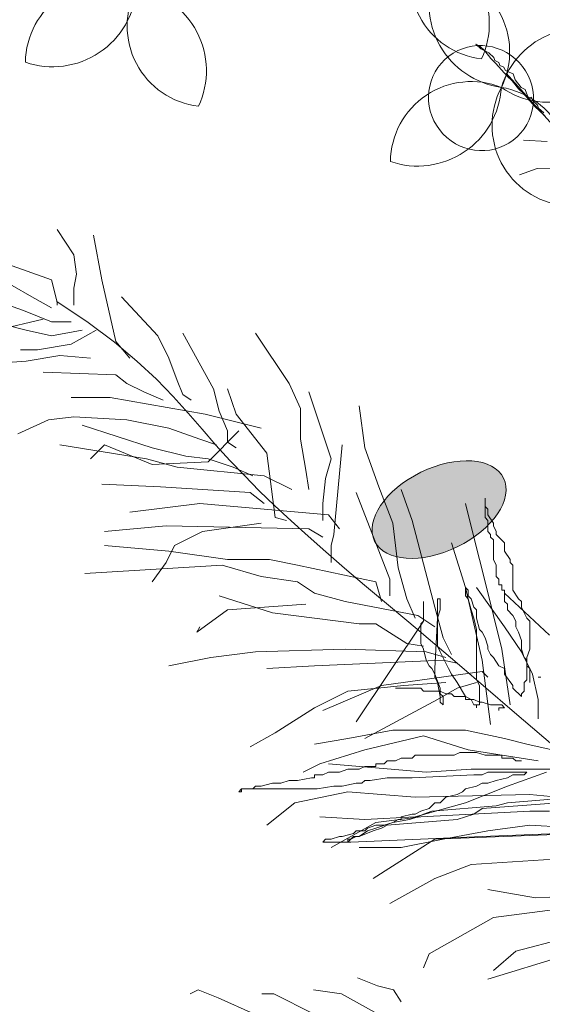
# Model space of a CAD drawing. Units: millimetres. Extents: x 595116 to 630915, y 909473 to 920225.
# Tile 100 of 134: x 629798.317 to 629803.095, y 919172.019 to 919181.018. Entities that reach past the tile are written whole.
import ezdxf

# ---------------------------------------------------------------- set-up
doc = ezdxf.new("R2010")
doc.units = ezdxf.units.MM
doc.layers.add('L-PLNT', color=85, linetype='Continuous', lineweight=13)

# ---------------------------------------------------------------- blocks, each defined once
blk = doc.blocks.new('A$C4FB75ABC')
for p, q in [((1.9382, 4.6431), (1.9285, 4.6477)), ((1.9285, 4.6477), (1.9408, 4.6359)), ((1.9506, 4.6313), (1.9382, 4.6431)), ((1.9408, 4.6359), (1.9506, 4.6313)), ((1.9603, 4.6267), (1.9506, 4.6313)), ((1.9506, 4.6313), (1.9655, 4.6124)), ((1.9726, 4.6149), (1.9603, 4.6267)), ((1.9655, 4.6124), (1.9778, 4.6006)), ((1.9752, 4.6078), (1.9726, 4.6149)), ((1.985, 4.6032), (1.9752, 4.6078)), ((1.9876, 4.596), (1.985, 4.6032)), ((1.9778, 4.6006), (2.0051, 4.5699)), ((1.9973, 4.5914), (1.9876, 4.596)), ((1.9999, 4.5842), (1.9973, 4.5914)), ((2.0097, 4.5796), (1.9999, 4.5842)), ((2.0194, 4.575), (2.0097, 4.5796)), ((2.1238, 4.4424), (2.0025, 4.577)), ((2.0051, 4.5699), (2.0174, 4.5581)), ((2.0174, 4.5581), (2.0323, 4.5391)), ((2.0246, 4.5607), (2.0194, 4.575)), ((2.0395, 4.5417), (2.0246, 4.5607)), ((2.0323, 4.5391), (2.0447, 4.5274)), ((2.0493, 4.5371), (2.0395, 4.5417)), ((2.057, 4.5156), (2.0493, 4.5371)), ((2.0447, 4.5274), (2.0719, 4.4967)), ((2.0642, 4.5182), (2.057, 4.5156)), ((2.0668, 4.511), (2.0642, 4.5182)), ((2.0791, 4.4992), (2.0668, 4.511)), ((2.0719, 4.4967), (2.0966, 4.4731)), ((2.0817, 4.4921), (2.0791, 4.4992)), ((2.094, 4.4803), (2.0817, 4.4921)), ((2.1029, 4.4105), (2.0449, 4.414)), ((2.0779, 4.3448), (2.0349, 4.3293)), ((2.1261, 4.346), (2.0779, 4.3448)), ((0.9087, 4.1962), (0.9496, 4.1349)), ((0.9973, 4.1826), (1.0177, 4.0736)), ((0.9496, 4.1349), (0.9564, 4.0872)), ((0.7997, 4.1076), (0.8951, 4.0736)), ((0.9564, 4.0872), (0.9496, 4.0532)), ((0.8474, 4.0327), (0.7997, 4.06)), ((0.8951, 4.0736), (0.9087, 4.0191)), ((0.9496, 4.0532), (0.9496, 4.0123)), ((1.0177, 4.0736), (1.0518, 3.9238)), ((0.8951, 4.0055), (0.8474, 4.0327)), ((1.0654, 4.0327), (1.154, 3.9374)), ((0.752, 4.0259), (0.827, 3.9987)), ((0.9842, 3.9699), (0.9085, 4.0207)), ((0.9087, 4.0191), (0.9087, 4.0123)), ((0.827, 3.9987), (0.8951, 3.9715)), ((0.8746, 3.9783), (0.7316, 3.9442)), ((0.8338, 3.951), (0.7793, 3.9647)), ((0.8951, 3.9715), (0.9428, 3.9715)), ((1.0487, 3.9217), (0.9842, 3.9699)), ((0.8951, 3.9374), (0.8338, 3.951)), ((0.97, 3.951), (0.8951, 3.9374)), ((1.0041, 3.951), (0.9428, 3.917)), ((1.154, 3.9374), (1.1812, 3.8829)), ((1.2153, 3.9442), (1.2902, 3.808)), ((1.3924, 3.9442), (1.4742, 3.8217)), ((0.9428, 3.917), (0.861, 3.9034)), ((1.1035, 3.8758), (1.0487, 3.9217)), ((1.0518, 3.9238), (1.0858, 3.8829)), ((0.861, 3.9034), (0.8201, 3.9034)), ((0.9155, 3.8897), (0.8338, 3.8761)), ((0.9905, 3.8829), (0.9155, 3.8897)), ((0.8338, 3.8761), (0.7452, 3.8693)), ((1.1506, 3.8319), (1.1035, 3.8758)), ((1.1812, 3.8829), (1.2017, 3.8285)), ((0.8746, 3.8489), (1.0518, 3.8421)), ((1.0518, 3.8421), (1.079, 3.8217)), ((1.079, 3.8217), (1.1199, 3.8012)), ((1.1917, 3.7897), (1.1506, 3.8319)), ((1.2017, 3.8285), (1.2153, 3.7944)), ((1.4742, 3.8217), (1.5014, 3.7604)), ((1.1199, 3.8012), (1.1676, 3.7808)), ((1.2284, 3.7492), (1.1917, 3.7897)), ((1.2153, 3.7944), (1.2357, 3.7808)), ((1.2902, 3.808), (1.3039, 3.7536)), ((1.3243, 3.808), (1.3447, 3.7467)), ((1.5219, 3.8012), (1.5764, 3.6378)), ((0.9428, 3.7876), (1.0382, 3.7876)), ((1.0382, 3.7876), (1.2698, 3.7467)), ((1.6445, 3.7672), (1.6581, 3.665)), ((1.2625, 3.7099), (1.2284, 3.7492)), ((1.2698, 3.7467), (1.4061, 3.7127)), ((1.3039, 3.7536), (1.3243, 3.7059)), ((1.3447, 3.7467), (1.4197, 3.6514)), ((1.5014, 3.7604), (1.5014, 3.6855)), ((0.8133, 3.6991), (0.8883, 3.7331)), ((0.8883, 3.7331), (0.9496, 3.7399)), ((0.9496, 3.7399), (1.079, 3.7331)), ((0.97, 3.7195), (1.1403, 3.665)), ((1.079, 3.7331), (1.1812, 3.7127)), ((1.1812, 3.7127), (1.2562, 3.6855)), ((1.2959, 3.6716), (1.2625, 3.7099)), ((1.3515, 3.7059), (1.2766, 3.631)), ((1.3243, 3.7059), (1.3243, 3.6787)), ((0.9155, 3.6718), (1.1267, 3.6378)), ((1.0245, 3.6718), (0.9905, 3.6378)), ((1.1403, 3.6242), (1.0245, 3.6718)), ((1.2562, 3.6855), (1.297, 3.6718)), ((1.3299, 3.6341), (1.2959, 3.6716)), ((1.3243, 3.6787), (1.3447, 3.665)), ((1.5014, 3.6855), (1.5151, 3.6106)), ((1.6036, 3.6718), (1.5832, 3.4539)), ((1.1403, 3.665), (1.2221, 3.6446)), ((1.2221, 3.6446), (1.2766, 3.6378)), ((1.4197, 3.6514), (1.4401, 3.4948)), ((1.6581, 3.665), (1.6922, 3.5697)), ((1.1267, 3.6378), (1.2017, 3.6174)), ((1.2766, 3.631), (1.1403, 3.6242)), ((1.2766, 3.6378), (1.3379, 3.6174)), ((1.365, 3.5971), (1.3299, 3.6341)), ((1.5764, 3.6378), (1.5627, 3.5901)), ((1.2017, 3.6174), (1.4129, 3.5969)), ((1.3379, 3.6174), (1.3856, 3.5969)), ((1.4014, 3.5604), (1.365, 3.5971)), ((1.4129, 3.5969), (1.481, 3.5629)), ((1.5151, 3.6106), (1.5219, 3.5629)), ((1.0177, 3.5765), (1.1608, 3.5697)), ((1.5627, 3.5901), (1.5559, 3.5288)), ((1.1608, 3.5697), (1.3788, 3.5561)), ((1.3788, 3.5561), (1.4129, 3.5288)), ((1.4393, 3.5237), (1.4014, 3.5604)), ((1.6377, 3.5561), (1.7194, 3.345)), ((1.6922, 3.5697), (1.7263, 3.4812)), ((1.7467, 3.5629), (1.7739, 3.488)), ((1.0858, 3.5084), (1.2562, 3.5288)), ((1.2562, 3.5288), (1.5696, 3.5016)), ((1.5559, 3.5288), (1.5559, 3.488)), ((1.9034, 3.5288), (1.9238, 3.4471)), ((1.9511, 3.4948), (1.9511, 3.5425)), ((1.9511, 3.5425), (1.9511, 3.522)), ((1.4788, 3.4868), (1.4393, 3.5237)), ((1.5696, 3.5016), (1.5968, 3.4676)), ((1.9511, 3.522), (1.9579, 3.5152)), ((1.9579, 3.5152), (1.9579, 3.5016)), ((1.9579, 3.5016), (1.9715, 3.4812)), ((1.4061, 3.4812), (1.263, 3.4608)), ((1.4401, 3.4948), (1.4674, 3.488)), ((1.5201, 3.4494), (1.4788, 3.4868)), ((1.7263, 3.4812), (1.7399, 3.3722)), ((1.7739, 3.488), (1.8285, 3.2769)), ((1.9579, 3.488), (1.9511, 3.4948)), ((1.9579, 3.4608), (1.9579, 3.488)), ((1.9715, 3.4812), (1.9715, 3.4744)), ((1.0245, 3.4608), (1.1744, 3.4744)), ((1.1744, 3.4744), (1.5219, 3.4676)), ((1.263, 3.4608), (1.1949, 3.4267)), ((1.5219, 3.4676), (1.5559, 3.4471)), ((1.5832, 3.4539), (1.5764, 3.4267)), ((1.9647, 3.4539), (1.9579, 3.4608)), ((1.9647, 3.4471), (1.9647, 3.4539)), ((1.9715, 3.4744), (1.9783, 3.4608)), ((1.9783, 3.4608), (1.9783, 3.4539)), ((1.9783, 3.4539), (1.9988, 3.4335)), ((1.5633, 3.4112), (1.5201, 3.4494)), ((1.8693, 3.4335), (1.9034, 3.3246)), ((1.9238, 3.4471), (1.9511, 3.3382)), ((1.9715, 3.4403), (1.9647, 3.4471)), ((1.9715, 3.3927), (1.9715, 3.4403)), ((1.9988, 3.4335), (1.9988, 3.4131)), ((1.0245, 3.4267), (1.1812, 3.4131)), ((1.1949, 3.4267), (1.1744, 3.3858)), ((1.1812, 3.4131), (1.3243, 3.3927)), ((1.6088, 3.3721), (1.5633, 3.4112)), ((1.5764, 3.4267), (1.5764, 3.3858)), ((1.9988, 3.4131), (2.0124, 3.3927)), ((1.1744, 3.3858), (1.1403, 3.3382)), ((1.3243, 3.3927), (1.4265, 3.3927)), ((1.4265, 3.3927), (1.4946, 3.379)), ((1.9783, 3.379), (1.9715, 3.3927)), ((2.0124, 3.3927), (2.0124, 3.3858)), ((2.0124, 3.3858), (2.0192, 3.379)), ((0.9768, 3.3586), (1.3107, 3.379)), ((1.3107, 3.379), (1.4061, 3.3518)), ((1.4946, 3.379), (1.6854, 3.3382)), ((1.6577, 3.3307), (1.6088, 3.3721)), ((1.7399, 3.3722), (1.7603, 3.2973)), ((1.9783, 3.3518), (1.9783, 3.379)), ((2.0192, 3.379), (2.0192, 3.3178)), ((1.4061, 3.3518), (1.4946, 3.3382)), ((1.4946, 3.3382), (1.5355, 3.3109)), ((1.6854, 3.3382), (1.699, 3.2905)), ((1.7194, 3.345), (1.7194, 3.3041)), ((1.9511, 3.3382), (1.992, 3.1748)), ((1.9851, 3.345), (1.9783, 3.3518)), ((1.9851, 3.3314), (1.9851, 3.345)), ((1.5355, 3.3109), (1.6104, 3.2905)), ((1.7159, 3.2817), (1.6577, 3.3307)), ((1.9102, 3.3178), (1.9034, 3.3246)), ((1.9034, 3.3246), (1.9034, 3.3041)), ((1.9034, 3.3246), (1.9443, 3.1475)), ((1.9102, 3.3041), (1.9102, 3.3178)), ((1.9306, 3.3246), (1.9988, 3.2292)), ((1.992, 3.3314), (1.9851, 3.3314)), ((1.992, 3.3178), (1.992, 3.3314)), ((1.9988, 3.3178), (1.992, 3.3178)), ((1.9988, 3.2905), (1.9988, 3.3178)), ((1.9988, 3.3109), (2.1078, 3.2088)), ((2.0192, 3.3178), (2.0328, 3.2973)), ((1.3039, 3.3041), (1.4333, 3.2633)), ((1.6104, 3.2905), (1.7876, 3.2565)), ((1.7603, 3.2973), (1.7808, 3.2497)), ((1.8012, 3.2429), (1.8012, 3.2905)), ((1.8012, 3.2905), (1.8012, 3.2429)), ((1.8421, 3.2973), (1.8353, 3.2973)), ((1.8353, 3.2973), (1.8353, 3.2497)), ((1.8421, 3.2701), (1.8421, 3.2973)), ((1.9034, 3.3041), (1.9102, 3.2973)), ((1.917, 3.2973), (1.9102, 3.3041)), ((1.9102, 3.2973), (1.917, 3.2701)), ((1.9238, 3.2769), (1.917, 3.2973)), ((2.0056, 3.2837), (1.9988, 3.2905)), ((2.0328, 3.2973), (2.0396, 3.2905)), ((2.0396, 3.2905), (2.0396, 3.2769)), ((1.3243, 3.2701), (1.2494, 3.2156)), ((1.5151, 3.2837), (1.3243, 3.2701)), ((1.4333, 3.2633), (1.6445, 3.236)), ((1.7906, 3.2188), (1.7159, 3.2817)), ((1.8285, 3.2769), (1.8489, 3.202)), ((1.8353, 3.2497), (1.8421, 3.2701)), ((1.917, 3.2701), (1.9238, 3.2497)), ((1.9306, 3.2701), (1.9238, 3.2769)), ((1.9306, 3.2497), (1.9306, 3.2701)), ((2.0056, 3.2701), (2.0056, 3.2837)), ((2.0192, 3.2565), (2.0056, 3.2701)), ((2.0396, 3.2769), (2.0465, 3.2633)), ((2.0465, 3.2633), (2.0533, 3.2497)), ((1.8012, 3.2429), (1.6377, 2.9977)), ((1.7876, 3.2565), (1.8285, 3.2292)), ((1.7944, 3.236), (1.8012, 3.2429)), ((1.8353, 3.2497), (1.8285, 3.1271)), ((1.8353, 3.1816), (1.8353, 3.2497)), ((1.9238, 3.2497), (1.9306, 3.2224)), ((1.9375, 3.2224), (1.9306, 3.2497)), ((2.026, 3.2429), (2.0192, 3.2565)), ((2.026, 3.2292), (2.026, 3.2429)), ((2.0533, 3.2497), (2.0601, 3.2429)), ((2.0601, 3.2429), (2.0601, 3.1748)), ((1.2494, 3.2156), (1.2562, 3.2292)), ((1.6445, 3.236), (1.6854, 3.236)), ((1.6854, 3.236), (1.7603, 3.1884)), ((1.8887, 3.1355), (1.7906, 3.2188)), ((1.7944, 3.1884), (1.7944, 3.236)), ((1.9306, 3.2224), (1.9306, 3.0999)), ((1.9443, 3.2156), (1.9375, 3.2224)), ((1.9511, 3.202), (1.9443, 3.2156)), ((1.9988, 3.2292), (2.0396, 3.1679)), ((2.0328, 3.2156), (2.026, 3.2292)), ((2.0396, 3.1952), (2.0328, 3.2156)), ((1.8489, 3.202), (1.8693, 3.1611)), ((1.9579, 3.1816), (1.9511, 3.202)), ((2.0396, 3.1748), (2.0396, 3.1952)), ((1.2834, 3.1543), (1.3924, 3.1679)), ((1.3924, 3.1679), (1.6104, 3.1748)), ((1.6104, 3.1748), (1.808, 3.1679)), ((1.7603, 3.1884), (1.8012, 3.1816)), ((1.8012, 3.1748), (1.7944, 3.1884)), ((1.808, 3.1475), (1.8012, 3.1748)), ((1.808, 3.1679), (1.8557, 3.1543)), ((1.8421, 3.1679), (1.8353, 3.1816)), ((1.8557, 3.1407), (1.8421, 3.1679)), ((1.9579, 3.1748), (1.9579, 3.1816)), ((1.9647, 3.1611), (1.9579, 3.1748)), ((1.992, 3.1748), (2.0124, 3.0386)), ((2.0465, 3.1543), (2.0396, 3.1748)), ((2.0396, 3.1679), (2.0669, 3.1135)), ((2.0601, 3.1748), (2.0533, 3.1543)), ((1.1812, 3.1339), (1.2834, 3.1543)), ((1.5355, 3.1339), (1.8489, 3.1475)), ((1.8148, 3.1339), (1.808, 3.1475)), ((1.8489, 3.1475), (1.883, 3.1407)), ((1.8625, 3.1271), (1.8557, 3.1407)), ((1.9443, 3.1475), (1.9647, 2.9909)), ((1.9715, 3.1543), (1.9647, 3.1611)), ((1.9851, 3.1339), (1.9715, 3.1543)), ((2.0533, 3.1475), (2.0465, 3.1543)), ((2.0533, 3.1543), (2.0533, 3.0999)), ((2.0533, 3.1339), (2.0533, 3.1475)), ((1.4197, 3.1271), (1.5355, 3.1339)), ((1.699, 3.0862), (1.9443, 3.1203)), ((1.8216, 3.1271), (1.8148, 3.1339)), ((1.8285, 3.1135), (1.8216, 3.1271)), ((1.8285, 3.1271), (1.8285, 3.1067)), ((1.8693, 3.1135), (1.8625, 3.1271)), ((2.0174, 3.0255), (1.8887, 3.1355)), ((1.9443, 3.1203), (1.9579, 3.1067)), ((1.9988, 3.1271), (1.9851, 3.1339)), ((1.9988, 3.1135), (1.9988, 3.1271)), ((2.0601, 3.1271), (2.0533, 3.1339)), ((2.0601, 3.093), (2.0601, 3.1271)), ((1.8557, 3.093), (1.7535, 3.0862)), ((1.8421, 3.0794), (1.8285, 3.1135)), ((1.8285, 3.1067), (1.8353, 3.093)), ((1.8353, 3.093), (1.8421, 3.059)), ((1.883, 3.093), (1.8693, 3.1135)), ((1.9034, 3.059), (1.883, 3.093)), ((1.883, 3.0794), (1.9306, 3.093)), ((1.9306, 3.0999), (1.9375, 3.0862)), ((2.0192, 3.0862), (1.9988, 3.1135)), ((2.0533, 3.0999), (2.0465, 3.093)), ((2.0465, 3.093), (2.0465, 3.0726)), ((2.0669, 3.1135), (2.0805, 3.0522)), ((2.0873, 3.1067), (2.0805, 3.1067)), ((1.6173, 3.0726), (1.5355, 3.0318)), ((1.5559, 3.0249), (1.699, 3.0862)), ((1.7535, 3.0862), (1.6173, 3.0726)), ((1.7331, 3.0794), (1.7944, 3.0794)), ((1.7944, 3.0794), (1.8012, 3.0726)), ((1.8012, 3.0726), (1.8421, 3.0726)), ((1.8353, 3.0522), (1.883, 3.0794)), ((1.8421, 3.0658), (1.8421, 3.0794)), ((1.8421, 3.0726), (1.8557, 3.0658)), ((1.9375, 3.0862), (1.9375, 3.0386)), ((2.0192, 3.0794), (2.0192, 3.0862)), ((2.0396, 3.059), (2.0192, 3.0794)), ((2.0465, 3.0726), (2.0396, 3.0658)), ((1.6581, 2.9569), (1.8353, 3.0522)), ((1.8489, 3.059), (1.8421, 3.0658)), ((1.8421, 3.059), (1.8421, 3.0454)), ((1.8421, 3.0454), (1.8489, 3.0386)), ((1.8489, 3.0386), (1.8489, 3.059)), ((1.8557, 3.0658), (1.8693, 3.0658)), ((1.8693, 3.0658), (1.8761, 3.059)), ((1.8761, 3.059), (1.9034, 3.059)), ((1.917, 3.0522), (1.9034, 3.059)), ((1.9034, 3.059), (1.9034, 3.0522)), ((1.9034, 3.0522), (1.9238, 3.0522)), ((1.9238, 3.0386), (1.917, 3.0522)), ((1.9238, 3.0522), (1.9375, 3.0454)), ((1.9375, 3.0454), (1.9443, 3.0454)), ((1.9443, 3.0454), (1.9647, 3.0386)), ((2.0396, 3.0658), (2.0396, 3.059)), ((2.0805, 3.0522), (2.0805, 3.0045)), ((1.5355, 3.0318), (1.4401, 2.9705)), ((1.9306, 3.0386), (1.9238, 3.0386)), ((1.9375, 3.0386), (1.9306, 3.0386)), ((1.9306, 3.0386), (1.9306, 3.0318)), ((1.9306, 3.0318), (1.9306, 3.0386)), ((1.9647, 3.0386), (1.992, 3.0386)), ((1.9988, 3.0318), (1.9851, 3.0318)), ((1.9851, 3.0318), (1.9851, 3.0249)), ((1.992, 3.0386), (1.9988, 3.0318)), ((2.1835, 2.8826), (2.0174, 3.0255)), ((1.6173, 2.9569), (1.7263, 2.9773)), ((1.7263, 2.9773), (1.9034, 2.9773)), ((1.9034, 2.9773), (1.9988, 2.9569)), ((1.4401, 2.9705), (1.3788, 2.9364)), ((1.5355, 2.9432), (1.6173, 2.9569)), ((1.8012, 2.9637), (1.6581, 2.9296)), ((1.9102, 2.9296), (1.8012, 2.9637)), ((1.9988, 2.9569), (2.0533, 2.9432)), ((1.6581, 2.9296), (1.5491, 2.8956)), ((2.0805, 2.9024), (1.9102, 2.9296)), ((2.0533, 2.9432), (2.1146, 2.9296)), ((1.7126, 2.9024), (1.7058, 2.8956)), ((1.7331, 2.9024), (1.7126, 2.9024)), ((1.7467, 2.9092), (1.7331, 2.9024)), ((1.7739, 2.9092), (1.7467, 2.9092)), ((1.7808, 2.916), (1.7739, 2.9092)), ((1.8761, 2.916), (1.7808, 2.916)), ((1.8898, 2.9228), (1.8761, 2.916)), ((1.9306, 2.9228), (1.8898, 2.9228)), ((1.9511, 2.916), (1.9306, 2.9228)), ((1.992, 2.916), (1.9511, 2.916)), ((1.992, 2.9092), (1.992, 2.916)), ((2.0192, 2.9092), (1.992, 2.9092)), ((2.026, 2.9024), (2.0192, 2.9092)), ((2.0396, 2.9024), (2.026, 2.9024)), ((1.5491, 2.8956), (1.5082, 2.8751)), ((1.5696, 2.8956), (1.808, 2.8751)), ((1.6173, 2.882), (1.5968, 2.8751)), ((1.6445, 2.882), (1.6173, 2.882)), ((1.6581, 2.8888), (1.6445, 2.882)), ((1.6854, 2.8888), (1.6581, 2.8888)), ((1.6854, 2.8956), (1.6854, 2.8888)), ((1.7058, 2.8956), (1.6854, 2.8956)), ((1.808, 2.8751), (1.917, 2.882)), ((1.917, 2.882), (2.1146, 2.882)), ((1.4742, 2.8547), (1.4537, 2.8479)), ((1.4946, 2.8547), (1.4742, 2.8547)), ((1.5287, 2.8615), (1.4946, 2.8547)), ((1.5355, 2.8615), (1.5287, 2.8615)), ((1.5559, 2.8683), (1.5355, 2.8683)), ((1.5355, 2.8683), (1.5355, 2.8615)), ((1.5696, 2.8751), (1.5559, 2.8683)), ((1.5968, 2.8751), (1.5696, 2.8751)), ((1.6513, 2.8479), (1.6581, 2.8547)), ((1.6581, 2.8547), (1.6718, 2.8547)), ((1.6718, 2.8547), (1.7126, 2.8615)), ((1.7126, 2.8615), (1.7739, 2.8615)), ((1.7739, 2.8615), (1.9238, 2.8683)), ((1.9238, 2.8683), (1.9443, 2.8683)), ((1.9443, 2.8683), (1.9579, 2.8751)), ((1.9579, 2.8751), (2.0533, 2.8751)), ((1.9783, 2.8547), (1.9579, 2.8479)), ((2.0056, 2.8615), (1.9783, 2.8547)), ((2.101, 2.8751), (2.0056, 2.8411)), ((2.0192, 2.8683), (2.0056, 2.8615)), ((2.0465, 2.8683), (2.0192, 2.8683)), ((2.0533, 2.8751), (2.0465, 2.8683)), ((1.3515, 2.8275), (1.3584, 2.8343)), ((1.3856, 2.8343), (1.3584, 2.8343)), ((1.3584, 2.8343), (1.3584, 2.8275)), ((1.3584, 2.8343), (1.5423, 2.8343)), ((1.3924, 2.8411), (1.3856, 2.8343)), ((1.4061, 2.8411), (1.3924, 2.8411)), ((1.4333, 2.8479), (1.4061, 2.8411)), ((1.4537, 2.8479), (1.4333, 2.8479)), ((1.5423, 2.8343), (1.5832, 2.8411)), ((1.5832, 2.8411), (1.6036, 2.8411)), ((1.6036, 2.8411), (1.6377, 2.8479)), ((1.6377, 2.8479), (1.6513, 2.8479)), ((1.9034, 2.8343), (1.8966, 2.8275)), ((1.9306, 2.8411), (1.9034, 2.8343)), ((2.0056, 2.8411), (1.9034, 2.8002)), ((1.9443, 2.8479), (1.9306, 2.8411)), ((1.9579, 2.8479), (1.9443, 2.8479)), ((1.3584, 2.8275), (1.3515, 2.8275)), ((1.4878, 2.8002), (1.6173, 2.8275)), ((1.6173, 2.8275), (1.7808, 2.8139)), ((1.7808, 2.8139), (2.0601, 2.8207)), ((1.8557, 2.8139), (1.8421, 2.8002)), ((1.883, 2.8207), (1.8557, 2.8139)), ((1.8966, 2.8275), (1.883, 2.8207)), ((2.1759, 2.8139), (2.0056, 2.8002)), ((2.0601, 2.8207), (2.1282, 2.8139)), ((1.4197, 2.7458), (1.4878, 2.8002)), ((1.9034, 2.8002), (1.7808, 2.7662)), ((1.8148, 2.7866), (1.7944, 2.7798)), ((1.8285, 2.8002), (1.8148, 2.7866)), ((1.9783, 2.7934), (1.8216, 2.7798)), ((1.8421, 2.8002), (1.8285, 2.8002)), ((1.9238, 2.773), (1.9443, 2.7866)), ((1.9443, 2.7866), (2.1282, 2.8002)), ((2.0056, 2.8002), (1.9783, 2.7934)), ((1.6581, 2.7594), (1.5491, 2.7662)), ((1.7808, 2.7662), (1.6581, 2.7594)), ((1.6854, 2.7526), (1.7944, 2.7662)), ((1.7126, 2.7458), (1.883, 2.7594)), ((1.7399, 2.7594), (1.7263, 2.7526)), ((1.7671, 2.7594), (1.7263, 2.7526)), ((1.7467, 2.7594), (1.7399, 2.7594)), ((1.7739, 2.773), (1.7467, 2.7662)), ((1.7467, 2.7662), (1.7467, 2.7594)), ((1.7876, 2.7662), (1.7671, 2.7594)), ((1.7808, 2.773), (1.7739, 2.773)), ((1.7944, 2.7798), (1.7808, 2.773)), ((1.8012, 2.773), (1.7876, 2.7662)), ((1.7944, 2.7662), (2.0601, 2.7798)), ((1.8216, 2.7798), (1.8012, 2.773)), ((1.883, 2.7594), (1.9034, 2.7662)), ((1.9034, 2.7662), (1.9238, 2.773)), ((2.0601, 2.7798), (2.1078, 2.7798)), ((1.5764, 2.6913), (1.6854, 2.7526)), ((1.6649, 2.739), (1.6581, 2.7321)), ((1.6854, 2.7458), (1.6649, 2.739)), ((1.6854, 2.739), (1.6649, 2.7321)), ((1.6786, 2.7321), (1.699, 2.739)), ((1.7263, 2.7526), (1.6854, 2.739)), ((1.7058, 2.7458), (1.6854, 2.7458)), ((1.699, 2.739), (1.7126, 2.7458)), ((1.7263, 2.7526), (1.7058, 2.7458)), ((2.0601, 2.7458), (1.9579, 2.7321)), ((2.1759, 2.739), (2.0601, 2.7458)), ((1.5627, 2.7117), (1.5559, 2.7049)), ((1.5764, 2.7117), (1.5627, 2.7117)), ((1.5968, 2.7185), (1.5764, 2.7117)), ((1.6036, 2.7185), (1.5968, 2.7185)), ((1.6309, 2.7253), (1.6036, 2.7185)), ((1.6309, 2.7185), (1.6173, 2.7049)), ((1.6173, 2.7049), (1.6173, 2.7117)), ((1.6173, 2.7117), (1.6241, 2.7117)), ((1.6241, 2.7117), (1.6377, 2.7185)), ((1.6241, 2.7049), (1.9443, 2.7185)), ((1.6377, 2.7321), (1.6309, 2.7253)), ((1.6445, 2.7185), (1.6309, 2.7185)), ((1.6581, 2.7321), (1.6377, 2.7321)), ((1.6377, 2.7185), (1.6445, 2.7185)), ((1.6649, 2.7321), (1.6445, 2.7185)), ((1.6445, 2.7185), (1.6786, 2.7321)), ((1.6786, 2.6164), (1.8285, 2.7117)), ((1.8489, 2.7117), (1.7467, 2.6913)), ((1.8285, 2.7117), (2.1691, 2.7253)), ((1.9579, 2.7321), (1.8489, 2.7117)), ((1.9443, 2.7185), (2.1282, 2.7253)), ((1.5559, 2.7049), (1.6241, 2.7049)), ((1.7467, 2.6913), (1.6445, 2.6913)), ((1.917, 2.6504), (2.2372, 2.6709)), ((1.8285, 2.6164), (1.917, 2.6504)), ((1.7194, 2.5551), (1.8285, 2.6164)), ((2.0737, 2.5687), (1.9579, 2.5891)), ((2.2032, 2.5755), (2.0737, 2.5687)), ((2.1282, 2.5415), (1.9715, 2.5211)), ((1.9715, 2.5211), (1.8148, 2.4325)), ((2.1555, 2.4734), (2.026, 2.4393)), ((1.8148, 2.4325), (1.8012, 2.3985)), ((2.1827, 2.4393), (1.9579, 2.3712)), ((2.026, 2.4393), (1.9715, 2.3917)), ((1.6891, 2.3546), (1.6405, 2.3741)), ((1.7279, 2.3449), (1.6891, 2.3546)), ((1.2522, 2.3449), (1.2328, 2.3352)), ((1.3008, 2.3255), (1.2522, 2.3449)), ((1.3881, 2.2867), (1.3008, 2.3255)), ((1.4367, 2.3352), (1.4075, 2.3352)), ((1.5337, 2.2867), (1.4367, 2.3352)), ((1.6017, 2.3352), (1.5337, 2.3449)), ((1.6891, 2.2867), (1.6017, 2.3352)), ((1.7473, 2.3158), (1.7279, 2.3449))]:
    blk.add_line(p, q)
blk = doc.blocks.new('A$C77972600')
h = blk.add_hatch(color=256)
edge = h.paths.add_edge_path()
edge.add_ellipse((4.1652, 1.933), major_axis=(0.1866, 0.0058), ratio=0.578492, start_angle=0, end_angle=360)
edge = h.paths.add_edge_path()
edge.add_ellipse((3.2944, 1.3586), major_axis=(0.1739, -0.0678), ratio=0.578492, start_angle=0, end_angle=360)
edge = h.paths.add_edge_path()
edge.add_ellipse((3.2064, 0.4835), major_axis=(0.1223, 0.141), ratio=0.578492, start_angle=0, end_angle=360)
edge = h.paths.add_edge_path()
edge.add_ellipse((2.6497, 0.127), major_axis=(0.1678, 0.0818), ratio=0.578492, start_angle=0, end_angle=360)
edge = h.paths.add_edge_path()
edge.add_ellipse((1.7252, 3.461), major_axis=(0.1678, 0.0818), ratio=0.578492, start_angle=0, end_angle=360)
edge = h.paths.add_edge_path()
edge.add_ellipse((2.1962, 2.8048), major_axis=(0.1678, 0.0818), ratio=0.578492, start_angle=0, end_angle=360)
edge = h.paths.add_edge_path()
edge.add_ellipse((1.7372, 2.8674), major_axis=(0.1866, 0.0058), ratio=0.578492, start_angle=0, end_angle=360)
edge = h.paths.add_edge_path()
edge.add_ellipse((3.2773, 2.4479), major_axis=(0.1739, -0.0678), ratio=0.578492, start_angle=0, end_angle=360)
edge = h.paths.add_edge_path()
edge.add_ellipse((3.6722, 2.9717), major_axis=(0.1739, -0.0678), ratio=0.578492, start_angle=0, end_angle=360)
edge = h.paths.add_edge_path()
edge.add_ellipse((2.9739, 2.7963), major_axis=(0.1739, -0.0678), ratio=0.578492, start_angle=0, end_angle=360)
edge = h.paths.add_edge_path()
edge.add_ellipse((4.8796, 2.4604), major_axis=(0.1678, 0.0818), ratio=0.578492, start_angle=0, end_angle=360)
edge = h.paths.add_edge_path()
edge.add_ellipse((4.2454, 2.1577), major_axis=(0.1678, 0.0818), ratio=0.578492, start_angle=0, end_angle=360)
edge = h.paths.add_edge_path()
edge.add_ellipse((4.4178, 2.4738), major_axis=(0.1678, 0.0818), ratio=0.578492, start_angle=0, end_angle=360)
edge = h.paths.add_edge_path()
edge.add_ellipse((4.3066, 3.973), major_axis=(0.1866, 0.0058), ratio=0.578492, start_angle=0, end_angle=360)
edge = h.paths.add_edge_path()
edge.add_ellipse((3.0828, 1.7149), major_axis=(0.1223, 0.141), ratio=0.578492, start_angle=0, end_angle=360)
edge = h.paths.add_edge_path()
edge.add_ellipse((4.1152, 4.8113), major_axis=(0.1678, 0.0818), ratio=0.578492, start_angle=0, end_angle=360)
edge = h.paths.add_edge_path()
edge.add_ellipse((4.4995, 4.8518), major_axis=(0.1223, 0.141), ratio=0.578492, start_angle=0, end_angle=360)
edge = h.paths.add_edge_path()
edge.add_ellipse((4.913, 5.2627), major_axis=(0.1678, 0.0818), ratio=0.578492, start_angle=0, end_angle=360)
edge = h.paths.add_edge_path()
edge.add_ellipse((5.0407, 4.562), major_axis=(0.1223, 0.141), ratio=0.578492, start_angle=0, end_angle=360)
edge = h.paths.add_edge_path()
edge.add_ellipse((4.6105, 4.3933), major_axis=(0.1223, 0.141), ratio=0.578492, start_angle=0, end_angle=360)
edge = h.paths.add_edge_path()
edge.add_ellipse((5.7235, 4.0986), major_axis=(0.1866, 0.0058), ratio=0.578492, start_angle=0, end_angle=360)
edge = h.paths.add_edge_path()
edge.add_ellipse((5.9977, 3.3249), major_axis=(0.1739, -0.0678), ratio=0.578492, start_angle=0, end_angle=360)
edge = h.paths.add_edge_path()
edge.add_ellipse((5.6486, 3.2372), major_axis=(0.1739, -0.0678), ratio=0.578492, start_angle=0, end_angle=360)
edge = h.paths.add_edge_path()
edge.add_ellipse((1.5981, 2.014), major_axis=(0.1678, 0.0818), ratio=0.578492, start_angle=0, end_angle=360)
edge = h.paths.add_edge_path()
edge.add_ellipse((2.2453, 5.0931), major_axis=(0.1678, 0.0818), ratio=0.578492, start_angle=0, end_angle=360)
edge = h.paths.add_edge_path()
edge.add_ellipse((2.073, 4.777), major_axis=(0.1678, 0.0818), ratio=0.578492, start_angle=0, end_angle=360)
edge = h.paths.add_edge_path()
edge.add_ellipse((1.2216, 4.5968), major_axis=(0.1866, 0.0058), ratio=0.578492, start_angle=0, end_angle=360)
edge = h.paths.add_edge_path()
edge.add_ellipse((1.6688, 4.0227), major_axis=(0.1866, 0.0058), ratio=0.578492, start_angle=0, end_angle=360)
edge = h.paths.add_edge_path()
edge.add_ellipse((1.253, 4.2244), major_axis=(0.1866, 0.0058), ratio=0.578492, start_angle=0, end_angle=360)
edge = h.paths.add_edge_path()
edge.add_ellipse((2.3257, 4.3332), major_axis=(0.1866, 0.0058), ratio=0.578492, start_angle=0, end_angle=360)
for centre, radius, start, end in [((2.7848, 1.5086), 0.2106, 152.1384, 263.3149), ((2.5621, 1.3915), 0.2185, 335.0581, 80.3951), ((2.8419, 1.442), 0.2185, 156.8071, 262.1441), ((2.6229, 1.3182), 0.2106, 333.8874, 85.0638), ((1.7838, 1.2884), 0.2106, 68.147, 179.3234), ((1.644, 1.4976), 0.2185, 251.0667, 356.4037), ((2.0484, 1.3855), 0.2106, 152.1384, 263.3149), ((1.8257, 1.2684), 0.2185, 335.0581, 80.3951), ((3.0209, 1.1614), 0.2185, 57.5868, 162.9238), ((2.9338, 1.3974), 0.2106, 234.6671, 345.8435), ((2.7336, 1.03), 0.2106, 68.147, 179.3234), ((2.5939, 1.2392), 0.2185, 251.0667, 356.4037), ((2.9982, 1.1271), 0.2106, 152.1384, 263.3149), ((2.7756, 1.0101), 0.2185, 335.0581, 80.3951)]:
    blk.add_arc(centre, radius, start, end)
blk.add_ellipse((2.7589, 1.1975), major_axis=(-0.0941, 0.1005), ratio=0.985729)
blk.add_ellipse((2.6497, 0.127), major_axis=(-0.1678, -0.0818), ratio=0.578492, start_param=-1.570796, end_param=4.712389)

msp = doc.modelspace()

# ---------------------------------------------------------------- block references
at = {"layer": 'L-PLNT'}
for name, p, xscale, yscale, zscale in [('A$C77972600', (629792.8437, 919176.0945), 3.512546757812034, 3.512546757812034, 3.512546757812034), ('A$C4FB75ABC', (629795.2477, 919163.3497), 3.753413438031968, 3.753413438031968, 3.753413438031968)]:
    msp.add_blockref(name, p, dxfattribs=dict(at, xscale=xscale, yscale=yscale, zscale=zscale))

doc.saveas('drawing.dxf')
